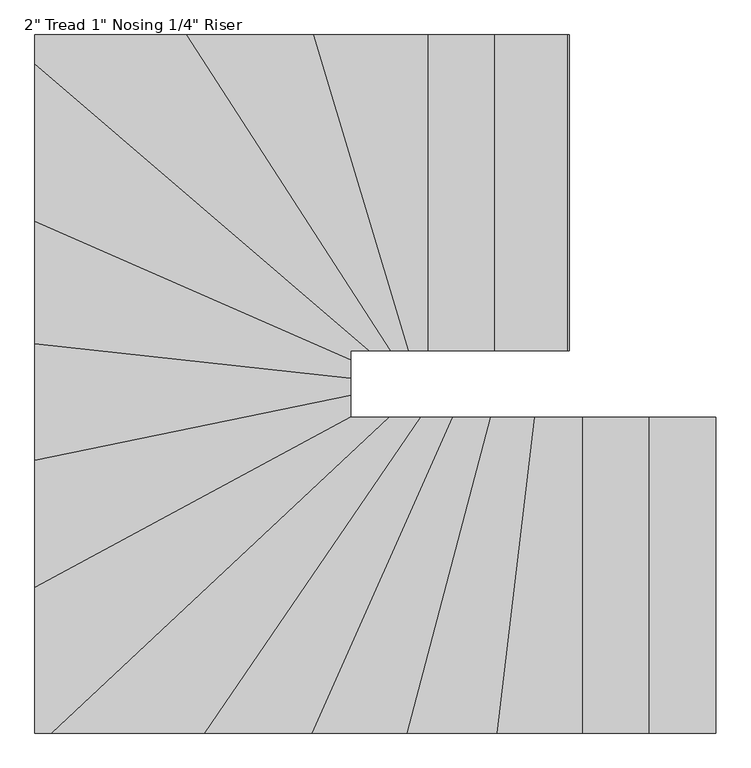
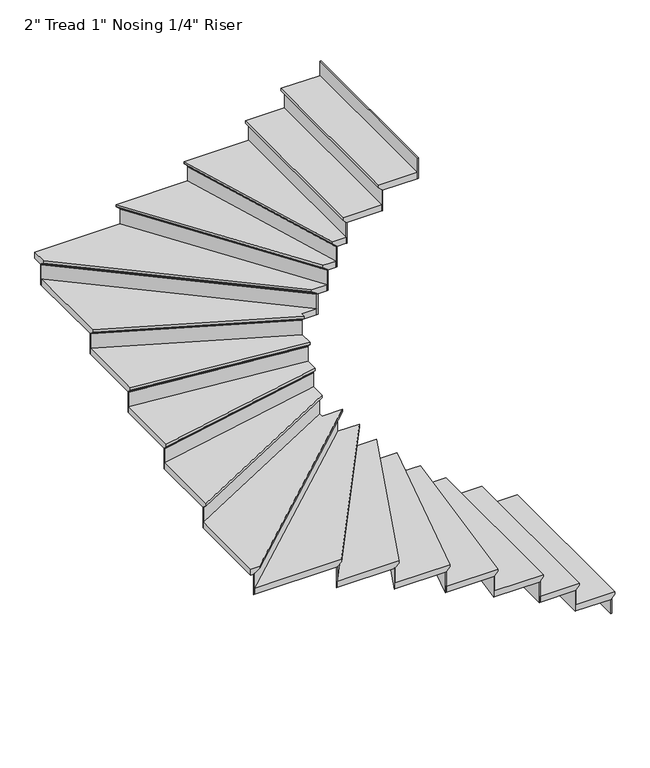
"""IFC4 building model written with IfcOpenShell, lengths in millimetres: stair flight geometry."""

from ifc_helpers import new_model, si_unit, origin, place, context, project, spatial, faceted_brep, source, transform, mapped, element, save


def stair_flight_ec2dc638(model_context):
    return source(origin(), model_context, "Body", "Brep", [
        faceted_brep([(-254.2696611, -2066.8011892, 150.2833333), (-254.2696611, -2066.8011892, 169.3333333), (-254.2696611, -3387.6011892, 169.3333333), (-254.2696611, -3387.6011892, 150.2833333), (-279.6696611, -2066.8011892, 124.8833333), (-279.6696611, -3387.6011892, 124.8833333), (-559.0696611, -2066.8011892, 169.3333333), (-559.0696611, -3387.6011892, 169.3333333), (-279.6696611, -3387.6011892, 118.5333333), (-559.0696611, -3387.6011892, 118.5333333), (-559.0696611, -2066.8011892, 118.5333333), (-279.6696611, -2066.8011892, 118.5333333)], [[[0, 1, 2, 3]], [[4, 0, 3, 5]], [[2, 1, 6, 7]], [[8, 9, 10, 11]], [[2, 7, 9, 8, 5, 3]], [[8, 11, 4, 5]], [[6, 1, 0, 4, 11, 10]], [[7, 6, 10, 9]]]),
        faceted_brep([(-279.6696611, -2066.8011892, 118.5333333), (-279.6696611, -2066.8011892, 0.0), (-286.0196611, -2066.8011892, 0.0), (-286.0196611, -2066.8011892, 118.5333333), (-279.6696611, -3387.6011892, 118.5333333), (-286.0196611, -3387.6011892, 118.5333333), (-286.0196611, -3387.6011892, 0.0), (-279.6696611, -3387.6011892, 0.0)], [[[0, 1, 2, 3]], [[4, 5, 6, 7]], [[1, 0, 4, 7]], [[2, 1, 7, 6]], [[3, 2, 6, 5]], [[0, 3, 5, 4]]]),
        faceted_brep([(-559.0696611, -2066.8011892, 287.8666667), (-559.0696611, -2066.8011892, 118.5333333), (-565.4196611, -2066.8011892, 118.5333333), (-565.4196611, -2066.8011892, 287.8666667), (-559.0696611, -3387.6011892, 287.8666667), (-565.4196611, -3387.6011892, 287.8666667), (-565.4196611, -3387.6011892, 118.5333333), (-559.0696611, -3387.6011892, 118.5333333)], [[[0, 1, 2, 3]], [[4, 5, 6, 7]], [[1, 0, 4, 7]], [[2, 1, 7, 6]], [[3, 2, 6, 5]], [[0, 3, 5, 4]]]),
        faceted_brep([(-533.6696611, -3387.6011892, 338.6666667), (-533.6696611, -2066.8011892, 338.6666667), (-838.4696611, -2066.8011892, 338.6666667), (-838.4696611, -3387.6011892, 338.6666667), (-559.0696611, -3387.6011892, 287.8666667), (-838.4696611, -3387.6011892, 287.8666667), (-838.4696611, -2066.8011892, 287.8666667), (-559.0696611, -2066.8011892, 287.8666667), (-559.0696611, -3387.6011892, 294.2166667), (-533.6696611, -3387.6011892, 319.6166667), (-559.0696611, -2066.8011892, 294.2166667), (-533.6696611, -2066.8011892, 319.6166667)], [[[0, 1, 2, 3]], [[4, 5, 6, 7]], [[0, 3, 5, 4, 8, 9]], [[4, 7, 10, 8]], [[2, 1, 11, 10, 7, 6]], [[3, 2, 6, 5]], [[11, 1, 0, 9]], [[10, 11, 9, 8]]]),
        faceted_brep([(-838.4696611, -2066.8011892, 457.2), (-838.4696611, -2066.8011892, 287.8666667), (-844.8196611, -2066.8011892, 287.8666667), (-844.8196611, -2066.8011892, 457.2), (-838.4696611, -3387.6011892, 457.2), (-844.8196611, -3387.6011892, 457.2), (-844.8196611, -3387.6011892, 287.8666667), (-838.4696611, -3387.6011892, 287.8666667)], [[[0, 1, 2, 3]], [[4, 5, 6, 7]], [[1, 0, 4, 7]], [[2, 1, 7, 6]], [[3, 2, 6, 5]], [[0, 3, 5, 4]]]),
        faceted_brep([(-813.0696611, -3387.6011892, 508.0), (-813.0696611, -2066.8011892, 508.0), (-1039.4980044, -2066.8011892, 508.0), (-1196.5994075, -3387.6011892, 508.0), (-838.4696611, -3387.6011892, 457.2), (-1196.5994075, -3387.6011892, 457.2), (-1039.4980044, -2066.8011892, 457.2), (-838.4696611, -2066.8011892, 457.2), (-838.4696611, -3387.6011892, 463.55), (-813.0696611, -3387.6011892, 488.95), (-838.4696611, -2066.8011892, 463.55), (-813.0696611, -2066.8011892, 488.95)], [[[0, 1, 2, 3]], [[4, 5, 6, 7]], [[0, 3, 5, 4, 8, 9]], [[4, 7, 10, 8]], [[2, 1, 11, 10, 7, 6]], [[3, 2, 6, 5]], [[11, 1, 0, 9]], [[10, 11, 9, 8]]]),
        faceted_brep([(-1039.4980044, -2066.8011892, 626.5333333), (-1039.4980044, -2066.8011892, 457.2), (-1045.8927656, -2066.8011892, 457.2), (-1045.8927656, -2066.8011892, 626.5333333), (-1196.5994075, -3387.6011892, 626.5333333), (-1202.9941687, -3387.6011892, 626.5333333), (-1202.9941687, -3387.6011892, 457.2), (-1196.5994075, -3387.6011892, 457.2)], [[[0, 1, 2, 3]], [[4, 5, 6, 7]], [[1, 0, 4, 7]], [[2, 1, 7, 6]], [[3, 2, 6, 5]], [[0, 3, 5, 4]]]),
        faceted_brep([(-1171.0203627, -3387.6011892, 677.3333333), (-1013.9189596, -2066.8011892, 677.3333333), (-1223.7629426, -2066.8011892, 677.3333333), (-1572.5174647, -3387.6011892, 677.3333333), (-1196.5994075, -3387.6011892, 626.5333333), (-1572.5174647, -3387.6011892, 626.5333333), (-1223.7629426, -2066.8011892, 626.5333333), (-1039.4980044, -2066.8011892, 626.5333333), (-1196.5994075, -3387.6011892, 632.8833333), (-1171.0203627, -3387.6011892, 658.2833333), (-1039.4980044, -2066.8011892, 632.8833333), (-1013.9189596, -2066.8011892, 658.2833333)], [[[0, 1, 2, 3]], [[4, 5, 6, 7]], [[0, 3, 5, 4, 8, 9]], [[4, 7, 10, 8]], [[2, 1, 11, 10, 7, 6]], [[3, 2, 6, 5]], [[11, 1, 0, 9]], [[10, 11, 9, 8]]]),
        faceted_brep([(-1223.7629426, -2066.8011892, 795.8666667), (-1223.7629426, -2066.8011892, 626.5333333), (-1230.3305782, -2066.8011892, 626.5333333), (-1230.3305782, -2066.8011892, 795.8666667), (-1572.5174647, -3387.6011892, 795.8666667), (-1579.0851003, -3387.6011892, 795.8666667), (-1579.0851003, -3387.6011892, 626.5333333), (-1572.5174647, -3387.6011892, 626.5333333)], [[[0, 1, 2, 3]], [[4, 5, 6, 7]], [[1, 0, 4, 7]], [[2, 1, 7, 6]], [[3, 2, 6, 5]], [[0, 3, 5, 4]]]),
        faceted_brep([(-1546.2469222, -3387.6011892, 846.6666667), (-1197.4924001, -2066.8011892, 846.6666667), (-1385.1880127, -2066.8011892, 846.6666667), (-1972.9542688, -3387.6011892, 846.6666667), (-1572.5174647, -3387.6011892, 795.8666667), (-1972.9542688, -3387.6011892, 795.8666667), (-1385.1880127, -2066.8011892, 795.8666667), (-1223.7629426, -2066.8011892, 795.8666667), (-1572.5174647, -3387.6011892, 802.2166667), (-1546.2469222, -3387.6011892, 827.6166667), (-1223.7629426, -2066.8011892, 802.2166667), (-1197.4924001, -2066.8011892, 827.6166667)], [[[0, 1, 2, 3]], [[4, 5, 6, 7]], [[0, 3, 5, 4, 8, 9]], [[4, 7, 10, 8]], [[2, 1, 11, 10, 7, 6]], [[3, 2, 6, 5]], [[11, 1, 0, 9]], [[10, 11, 9, 8]]]),
        faceted_brep([(-1385.1880127, -2066.8011892, 965.2), (-1385.1880127, -2066.8011892, 795.8666667), (-1392.1383826, -2066.8011892, 795.8666667), (-1392.1383826, -2066.8011892, 965.2), (-1972.9542688, -3387.6011892, 965.2), (-1979.9046387, -3387.6011892, 965.2), (-1979.9046387, -3387.6011892, 795.8666667), (-1972.9542688, -3387.6011892, 795.8666667)], [[[0, 1, 2, 3]], [[4, 5, 6, 7]], [[1, 0, 4, 7]], [[2, 1, 7, 6]], [[3, 2, 6, 5]], [[0, 3, 5, 4]]]),
        faceted_brep([(-1945.1527892, -3387.6011892, 1016.0), (-1357.3865331, -2066.8011892, 1016.0), (-1520.9558906, -2066.8011892, 1016.0), (-2423.9228406, -3387.6011892, 1016.0), (-1972.9542688, -3387.6011892, 965.2), (-2423.9228406, -3387.6011892, 965.2), (-1520.9558906, -2066.8011892, 965.2), (-1385.1880127, -2066.8011892, 965.2), (-1972.9542688, -3387.6011892, 971.55), (-1945.1527892, -3387.6011892, 996.95), (-1385.1880127, -2066.8011892, 971.55), (-1357.3865331, -2066.8011892, 996.95)], [[[0, 1, 2, 3]], [[4, 5, 6, 7]], [[0, 3, 5, 4, 8, 9]], [[4, 7, 10, 8]], [[2, 1, 11, 10, 7, 6]], [[3, 2, 6, 5]], [[11, 1, 0, 9]], [[10, 11, 9, 8]]]),
        faceted_brep([(-1520.9558906, -2066.8011892, 1134.5333333), (-1520.9558906, -2066.8011892, 965.2), (-1528.6479909, -2066.8011892, 965.2), (-1528.6479909, -2066.8011892, 1134.5333333), (-2423.9228406, -3387.6011892, 1134.5333333), (-2431.6149409, -3387.6011892, 1134.5333333), (-2431.6149409, -3387.6011892, 965.2), (-2423.9228406, -3387.6011892, 965.2)], [[[0, 1, 2, 3]], [[4, 5, 6, 7]], [[1, 0, 4, 7]], [[2, 1, 7, 6]], [[3, 2, 6, 5]], [[0, 3, 5, 4]]]),
        faceted_brep([(-2393.1544395, -3387.6011892, 1185.3333333), (-1490.1874895, -2066.8011892, 1185.3333333), (-1659.672175, -2066.8011892, 1185.3333333), (-3070.6127643, -3387.6011892, 1185.3333333), (-2423.9228406, -3387.6011892, 1134.5333333), (-3070.6127643, -3387.6011892, 1134.5333333), (-1659.672175, -2066.8011892, 1134.5333333), (-1520.9558906, -2066.8011892, 1134.5333333), (-2423.9228406, -3387.6011892, 1140.8833333), (-2393.1544395, -3387.6011892, 1166.2833333), (-1520.9558906, -2066.8011892, 1140.8833333), (-1490.1874895, -2066.8011892, 1166.2833333)], [[[0, 1, 2, 3]], [[4, 5, 6, 7]], [[0, 3, 5, 4, 8, 9]], [[4, 7, 10, 8]], [[2, 1, 11, 10, 7, 6]], [[3, 2, 6, 5]], [[11, 1, 0, 9]], [[10, 11, 9, 8]]]),
        faceted_brep([(-1659.672175, -2066.8011892, 1303.8666667), (-1659.672175, -2066.8011892, 1134.5333333), (-1668.9639232, -2066.8011892, 1134.5333333), (-1668.9639232, -2066.8011892, 1303.8666667), (-3070.6127643, -3387.6011892, 1303.8666667), (-3079.9045125, -3387.6011892, 1303.8666667), (-3079.9045125, -3387.6011892, 1134.5333333), (-3070.6127643, -3387.6011892, 1134.5333333)], [[[0, 1, 2, 3]], [[4, 5, 6, 7]], [[1, 0, 4, 7]], [[2, 1, 7, 6]], [[3, 2, 6, 5]], [[0, 3, 5, 4]]]),
        faceted_brep([(-3102.801353, -2748.4649023, 1354.6666667), (-3102.801353, -3387.6011892, 1354.6666667), (-3033.4457716, -3387.6011892, 1354.6666667), (-1622.5051823, -2066.8011892, 1354.6666667), (-1782.001353, -2066.8011892, 1354.6666667), (-1782.001353, -2035.767076, 1354.6666667), (-3102.801353, -3387.6011892, 1303.8666667), (-3102.801353, -2748.4649023, 1303.8666667), (-1782.001353, -2035.767076, 1303.8666667), (-1782.001353, -2066.8011892, 1303.8666667), (-1659.672175, -2066.8011892, 1303.8666667), (-3070.6127643, -3387.6011892, 1303.8666667), (-1659.672175, -2066.8011892, 1310.2166667), (-3070.6127643, -3387.6011892, 1310.2166667), (-1622.5051823, -2066.8011892, 1335.6166667), (-3033.4457716, -3387.6011892, 1335.6166667)], [[[0, 1, 2, 3, 4, 5]], [[6, 7, 8, 9, 10, 11]], [[1, 0, 7, 6]], [[11, 10, 12, 13]], [[5, 4, 9, 8]], [[0, 5, 8, 7]], [[14, 3, 2, 15]], [[12, 14, 15, 13]], [[2, 1, 6, 11, 13, 15]], [[4, 3, 14, 12, 10, 9]]]),
        faceted_brep([(-1782.001353, -2035.767076, 1473.2), (-1782.001353, -2035.767076, 1303.8666667), (-1782.001353, -2028.551611, 1303.8666667), (-1782.001353, -2028.551611, 1473.2), (-3102.801353, -2748.4649023, 1473.2), (-3102.801353, -2741.2494373, 1473.2), (-3102.801353, -2741.2494373, 1303.8666667), (-3102.801353, -2748.4649023, 1303.8666667)], [[[0, 1, 2, 3]], [[4, 5, 6, 7]], [[1, 0, 4, 7]], [[2, 1, 7, 6]], [[3, 2, 6, 5]], [[0, 3, 5, 4]]]),
        faceted_brep([(-3102.801353, -2777.3267624, 1524.0), (-1782.001353, -2064.628936, 1524.0), (-1782.001353, -1948.3283316, 1524.0), (-3102.801353, -2220.6109337, 1524.0), (-3102.801353, -2748.4649023, 1473.2), (-3102.801353, -2220.6109337, 1473.2), (-1782.001353, -1948.3283316, 1473.2), (-1782.001353, -2035.767076, 1473.2), (-3102.801353, -2748.4649023, 1479.55), (-3102.801353, -2777.3267624, 1504.95), (-1782.001353, -2035.767076, 1479.55), (-1782.001353, -2064.628936, 1504.95)], [[[0, 1, 2, 3]], [[4, 5, 6, 7]], [[0, 3, 5, 4, 8, 9]], [[4, 7, 10, 8]], [[2, 1, 11, 10, 7, 6]], [[3, 2, 6, 5]], [[11, 1, 0, 9]], [[10, 11, 9, 8]]]),
        faceted_brep([(-1782.001353, -1948.3283316, 1642.5333333), (-1782.001353, -1948.3283316, 1473.2), (-1782.001353, -1941.8448052, 1473.2), (-1782.001353, -1941.8448052, 1642.5333333), (-3102.801353, -2220.6109337, 1642.5333333), (-3102.801353, -2214.1274073, 1642.5333333), (-3102.801353, -2214.1274073, 1473.2), (-3102.801353, -2220.6109337, 1473.2)], [[[0, 1, 2, 3]], [[4, 5, 6, 7]], [[1, 0, 4, 7]], [[2, 1, 7, 6]], [[3, 2, 6, 5]], [[0, 3, 5, 4]]]),
        faceted_brep([(-3102.801353, -2246.5450393, 1693.3333333), (-1782.001353, -1974.2624372, 1693.3333333), (-1782.001353, -1876.7138033, 1693.3333333), (-3102.801353, -1733.6174886, 1693.3333333), (-3102.801353, -2220.6109337, 1642.5333333), (-3102.801353, -1733.6174886, 1642.5333333), (-1782.001353, -1876.7138033, 1642.5333333), (-1782.001353, -1948.3283316, 1642.5333333), (-3102.801353, -2220.6109337, 1648.8833333), (-3102.801353, -2246.5450393, 1674.2833333), (-1782.001353, -1948.3283316, 1648.8833333), (-1782.001353, -1974.2624372, 1674.2833333)], [[[0, 1, 2, 3]], [[4, 5, 6, 7]], [[0, 3, 5, 4, 8, 9]], [[4, 7, 10, 8]], [[2, 1, 11, 10, 7, 6]], [[3, 2, 6, 5]], [[11, 1, 0, 9]], [[10, 11, 9, 8]]]),
        faceted_brep([(-1782.001353, -1876.7138033, 1811.8666667), (-1782.001353, -1876.7138033, 1642.5333333), (-1782.001353, -1870.3266449, 1642.5333333), (-1782.001353, -1870.3266449, 1811.8666667), (-3102.801353, -1733.6174886, 1811.8666667), (-3102.801353, -1727.2303301, 1811.8666667), (-3102.801353, -1727.2303301, 1642.5333333), (-3102.801353, -1733.6174886, 1642.5333333)], [[[0, 1, 2, 3]], [[4, 5, 6, 7]], [[1, 0, 4, 7]], [[2, 1, 7, 6]], [[3, 2, 6, 5]], [[0, 3, 5, 4]]]),
        faceted_brep([(-3102.801353, -1759.1661224, 1862.6666667), (-1782.001353, -1902.2624372, 1862.6666667), (-1782.001353, -1797.5734199, 1862.6666667), (-3102.801353, -1218.9061969, 1862.6666667), (-3102.801353, -1733.6174886, 1811.8666667), (-3102.801353, -1218.9061969, 1811.8666667), (-1782.001353, -1797.5734199, 1811.8666667), (-1782.001353, -1876.7138033, 1811.8666667), (-3102.801353, -1733.6174886, 1818.2166667), (-3102.801353, -1759.1661224, 1843.6166667), (-1782.001353, -1876.7138033, 1818.2166667), (-1782.001353, -1902.2624372, 1843.6166667)], [[[0, 1, 2, 3]], [[4, 5, 6, 7]], [[0, 3, 5, 4, 8, 9]], [[4, 7, 10, 8]], [[2, 1, 11, 10, 7, 6]], [[3, 2, 6, 5]], [[11, 1, 0, 9]], [[10, 11, 9, 8]]]),
        faceted_brep([(-1782.001353, -1797.5734199, 1981.2), (-1782.001353, -1797.5734199, 1811.8666667), (-1782.001353, -1790.6407203, 1811.8666667), (-1782.001353, -1790.6407203, 1981.2), (-3102.801353, -1218.9061969, 1981.2), (-3102.801353, -1211.9734972, 1981.2), (-3102.801353, -1211.9734972, 1811.8666667), (-3102.801353, -1218.9061969, 1811.8666667)], [[[0, 1, 2, 3]], [[4, 5, 6, 7]], [[1, 0, 4, 7]], [[2, 1, 7, 6]], [[3, 2, 6, 5]], [[0, 3, 5, 4]]]),
        faceted_brep([(-3102.801353, -1246.6369954, 2032.0), (-1782.001353, -1825.3042184, 2032.0), (-1782.001353, -1787.4011892, 2032.0), (-1663.7103453, -1787.4011892, 2032.0), (-3102.801353, -554.2929231, 2032.0), (-3102.801353, -1218.9061969, 1981.2), (-3102.801353, -554.2929231, 1981.2), (-1663.7103453, -1787.4011892, 1981.2), (-1782.001353, -1787.4011892, 1981.2), (-1782.001353, -1797.5734199, 1981.2), (-3102.801353, -1218.9061969, 1987.55), (-3102.801353, -1246.6369954, 2012.95), (-1782.001353, -1797.5734199, 1987.55), (-1782.001353, -1825.3042184, 2012.95)], [[[0, 1, 2, 3, 4]], [[5, 6, 7, 8, 9]], [[0, 4, 6, 5, 10, 11]], [[5, 9, 12, 10]], [[2, 1, 13, 12, 9, 8]], [[4, 3, 7, 6]], [[13, 1, 0, 11]], [[12, 13, 11, 10]], [[3, 2, 8, 7]]]),
        faceted_brep([(-1663.7103453, -1787.4011892, 2150.5333333), (-1663.7103453, -1787.4011892, 1981.2), (-1653.951177, -1787.4011892, 1981.2), (-1653.951177, -1787.4011892, 2150.5333333), (-3102.801353, -554.2929231, 2150.5333333), (-3102.801353, -545.9306229, 2150.5333333), (-3102.801353, -545.9306229, 1981.2), (-3102.801353, -554.2929231, 1981.2)], [[[0, 1, 2, 3]], [[4, 5, 6, 7]], [[1, 0, 4, 7]], [[2, 1, 7, 6]], [[3, 2, 6, 5]], [[0, 3, 5, 4]]]),
        faceted_brep([(-2437.5518455, -466.6011892, 2201.3333333), (-3102.801353, -466.6011892, 2201.3333333), (-3102.801353, -587.7421239, 2201.3333333), (-1702.7470182, -1787.4011892, 2201.3333333), (-1582.7399849, -1787.4011892, 2201.3333333), (-3102.801353, -466.6011892, 2150.5333333), (-2437.5518455, -466.6011892, 2150.5333333), (-1582.7399849, -1787.4011892, 2150.5333333), (-1663.7103453, -1787.4011892, 2150.5333333), (-3102.801353, -554.2929231, 2150.5333333), (-1663.7103453, -1787.4011892, 2156.8833333), (-3102.801353, -554.2929231, 2156.8833333), (-1702.7470182, -1787.4011892, 2182.2833333), (-3102.801353, -587.7421239, 2182.2833333)], [[[0, 1, 2, 3, 4]], [[5, 6, 7, 8, 9]], [[1, 0, 6, 5]], [[9, 8, 10, 11]], [[4, 3, 12, 10, 8, 7]], [[0, 4, 7, 6]], [[12, 3, 2, 13]], [[10, 12, 13, 11]], [[2, 1, 5, 9, 11, 13]]]),
        faceted_brep([(-1582.7399849, -1787.4011892, 2319.8666667), (-1582.7399849, -1787.4011892, 2150.5333333), (-1575.1761296, -1787.4011892, 2150.5333333), (-1575.1761296, -1787.4011892, 2319.8666667), (-2437.5518455, -466.6011892, 2319.8666667), (-2429.9879902, -466.6011892, 2319.8666667), (-2429.9879902, -466.6011892, 2150.5333333), (-2437.5518455, -466.6011892, 2150.5333333)], [[[0, 1, 2, 3]], [[4, 5, 6, 7]], [[1, 0, 4, 7]], [[2, 1, 7, 6]], [[3, 2, 6, 5]], [[0, 3, 5, 4]]]),
        faceted_brep([(-2467.8072667, -466.6011892, 2370.6666667), (-1612.9954062, -1787.4011892, 2370.6666667), (-1512.2326122, -1787.4011892, 2370.6666667), (-1908.8741757, -466.6011892, 2370.6666667), (-2437.5518455, -466.6011892, 2319.8666667), (-1908.8741757, -466.6011892, 2319.8666667), (-1512.2326122, -1787.4011892, 2319.8666667), (-1582.7399849, -1787.4011892, 2319.8666667), (-2437.5518455, -466.6011892, 2326.2166667), (-2467.8072667, -466.6011892, 2351.6166667), (-1582.7399849, -1787.4011892, 2326.2166667), (-1612.9954062, -1787.4011892, 2351.6166667)], [[[0, 1, 2, 3]], [[4, 5, 6, 7]], [[0, 3, 5, 4, 8, 9]], [[4, 7, 10, 8]], [[2, 1, 11, 10, 7, 6]], [[3, 2, 6, 5]], [[11, 1, 0, 9]], [[10, 11, 9, 8]]]),
        faceted_brep([(-1512.2326122, -1787.4011892, 2489.2), (-1512.2326122, -1787.4011892, 2319.8666667), (-1505.6024625, -1787.4011892, 2319.8666667), (-1505.6024625, -1787.4011892, 2489.2), (-1908.8741757, -466.6011892, 2489.2), (-1902.244026, -466.6011892, 2489.2), (-1902.244026, -466.6011892, 2319.8666667), (-1908.8741757, -466.6011892, 2319.8666667)], [[[0, 1, 2, 3]], [[4, 5, 6, 7]], [[1, 0, 4, 7]], [[2, 1, 7, 6]], [[3, 2, 6, 5]], [[0, 3, 5, 4]]]),
        faceted_brep([(-1935.3947743, -466.6011892, 2540.0), (-1538.7532108, -1787.4011892, 2540.0), (-1432.2739925, -1787.4011892, 2540.0), (-1432.2739925, -466.6011892, 2540.0), (-1908.8741757, -466.6011892, 2489.2), (-1432.2739925, -466.6011892, 2489.2), (-1432.2739925, -1787.4011892, 2489.2), (-1512.2326122, -1787.4011892, 2489.2), (-1908.8741757, -466.6011892, 2495.55), (-1935.3947743, -466.6011892, 2520.95), (-1512.2326122, -1787.4011892, 2495.55), (-1538.7532108, -1787.4011892, 2520.95)], [[[0, 1, 2, 3]], [[4, 5, 6, 7]], [[0, 3, 5, 4, 8, 9]], [[4, 7, 10, 8]], [[2, 1, 11, 10, 7, 6]], [[3, 2, 6, 5]], [[11, 1, 0, 9]], [[10, 11, 9, 8]]]),
        faceted_brep([(-1432.2739925, -1787.4011892, 2658.5333333), (-1432.2739925, -1787.4011892, 2489.2), (-1425.9239925, -1787.4011892, 2489.2), (-1425.9239925, -1787.4011892, 2658.5333333), (-1432.2739925, -466.6011892, 2658.5333333), (-1425.9239925, -466.6011892, 2658.5333333), (-1425.9239925, -466.6011892, 2489.2), (-1432.2739925, -466.6011892, 2489.2)], [[[0, 1, 2, 3]], [[4, 5, 6, 7]], [[1, 0, 4, 7]], [[2, 1, 7, 6]], [[3, 2, 6, 5]], [[0, 3, 5, 4]]]),
        faceted_brep([(-1457.6739925, -466.6011892, 2709.3333333), (-1457.6739925, -1787.4011892, 2709.3333333), (-1152.8739925, -1787.4011892, 2709.3333333), (-1152.8739925, -466.6011892, 2709.3333333), (-1432.2739925, -466.6011892, 2658.5333333), (-1152.8739925, -466.6011892, 2658.5333333), (-1152.8739925, -1787.4011892, 2658.5333333), (-1432.2739925, -1787.4011892, 2658.5333333), (-1432.2739925, -466.6011892, 2664.8833333), (-1457.6739925, -466.6011892, 2690.2833333), (-1432.2739925, -1787.4011892, 2664.8833333), (-1457.6739925, -1787.4011892, 2690.2833333)], [[[0, 1, 2, 3]], [[4, 5, 6, 7]], [[0, 3, 5, 4, 8, 9]], [[4, 7, 10, 8]], [[2, 1, 11, 10, 7, 6]], [[3, 2, 6, 5]], [[11, 1, 0, 9]], [[10, 11, 9, 8]]]),
        faceted_brep([(-1152.8739925, -1787.4011892, 2827.8666667), (-1152.8739925, -1787.4011892, 2658.5333333), (-1146.5239925, -1787.4011892, 2658.5333333), (-1146.5239925, -1787.4011892, 2827.8666667), (-1152.8739925, -466.6011892, 2827.8666667), (-1146.5239925, -466.6011892, 2827.8666667), (-1146.5239925, -466.6011892, 2658.5333333), (-1152.8739925, -466.6011892, 2658.5333333)], [[[0, 1, 2, 3]], [[4, 5, 6, 7]], [[1, 0, 4, 7]], [[2, 1, 7, 6]], [[3, 2, 6, 5]], [[0, 3, 5, 4]]]),
        faceted_brep([(-873.4739925, -1787.4011892, 2997.2), (-873.4739925, -1787.4011892, 2827.8666667), (-867.1239925, -1787.4011892, 2827.8666667), (-867.1239925, -1787.4011892, 2997.2), (-873.4739925, -466.6011892, 2997.2), (-867.1239925, -466.6011892, 2997.2), (-867.1239925, -466.6011892, 2827.8666667), (-873.4739925, -466.6011892, 2827.8666667)], [[[0, 1, 2, 3]], [[4, 5, 6, 7]], [[1, 0, 4, 7]], [[2, 1, 7, 6]], [[3, 2, 6, 5]], [[0, 3, 5, 4]]]),
        faceted_brep([(-1178.2739925, -466.6011892, 2878.6666667), (-1178.2739925, -1787.4011892, 2878.6666667), (-873.4739925, -1787.4011892, 2878.6666667), (-873.4739925, -466.6011892, 2878.6666667), (-1152.8739925, -466.6011892, 2827.8666667), (-873.4739925, -466.6011892, 2827.8666667), (-873.4739925, -1787.4011892, 2827.8666667), (-1152.8739925, -1787.4011892, 2827.8666667), (-1152.8739925, -466.6011892, 2834.2166667), (-1178.2739925, -466.6011892, 2859.6166667), (-1152.8739925, -1787.4011892, 2834.2166667), (-1178.2739925, -1787.4011892, 2859.6166667)], [[[0, 1, 2, 3]], [[4, 5, 6, 7]], [[0, 3, 5, 4, 8, 9]], [[4, 7, 10, 8]], [[2, 1, 11, 10, 7, 6]], [[3, 2, 6, 5]], [[11, 1, 0, 9]], [[10, 11, 9, 8]]]),
    ])


if __name__ == "__main__":
    model = new_model("IFC4")
    model_context = context("Model", 3, world=origin())
    ifc_project = project(units=[si_unit("LENGTHUNIT", "METRE", prefix="MILLI")], contexts=[model_context])
    site = spatial("IfcSite", under=ifc_project)
    building = spatial("IfcBuilding", under=site)
    placement = place(None, origin())
    stair_flight_shape = stair_flight_ec2dc638(model_context)
    element("IfcStairFlight", 1, ObjectType="2\" Tread 1\" Nosing 1/4\" Riser", at=placement, inside=building, context=model_context, shape_type="MappedRepresentation", body=[
        mapped(stair_flight_shape, transform((0.0, 0.0, 0.0), x_axis=(1.0, 0.0, 0.0), y_axis=(0.0, 1.0, 0.0), z_axis=(0.0, 0.0, 1.0))),
    ])
    save(model, "model.ifc")
